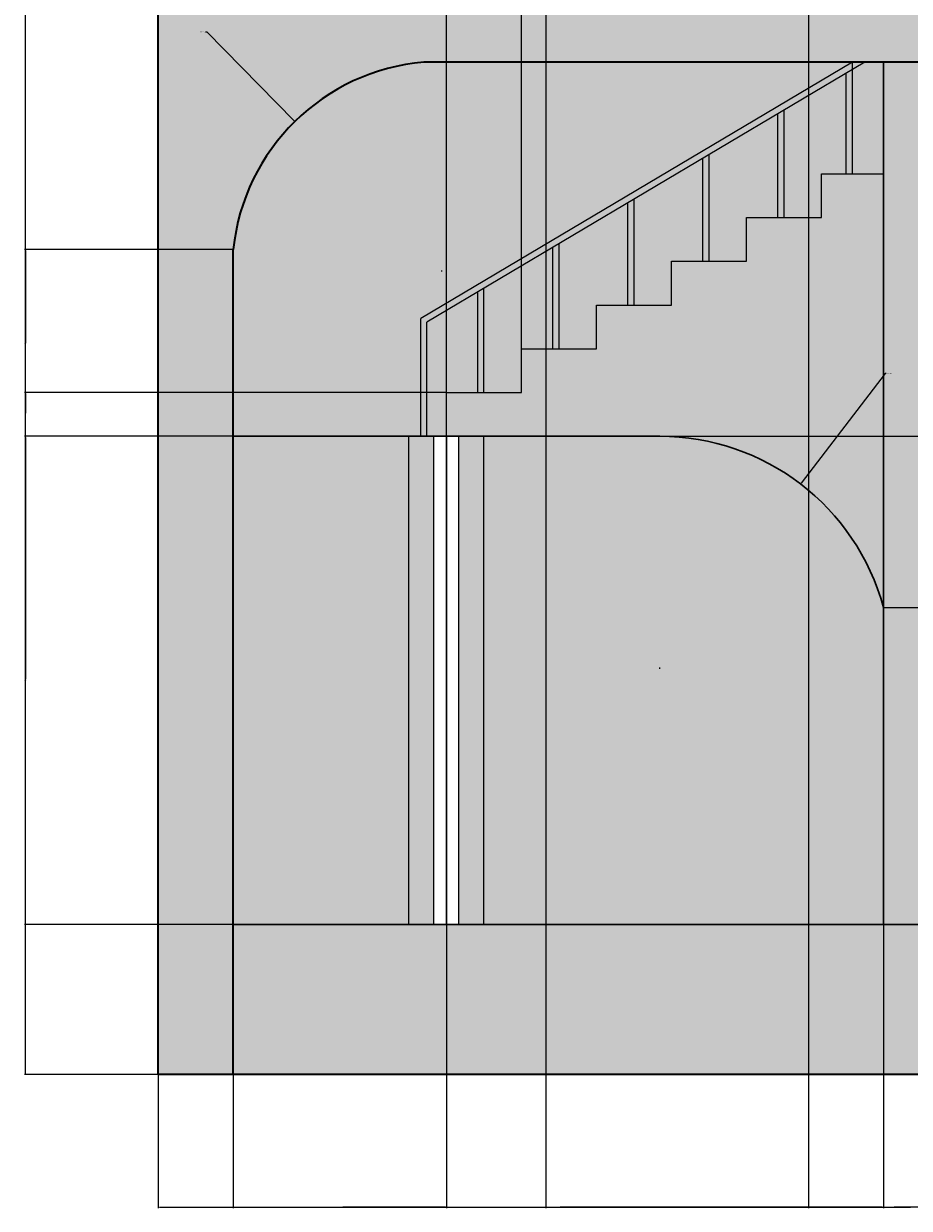
# Model space of a CAD drawing. Units: inches. Extents: x 2051 to 2334, y 814 to 1281.
# Tile 1 of 4: x 2051 to 2193, y 814 to 1003. Entities that reach past the tile are written whole.
import ezdxf

# ---------------------------------------------------------------- set-up
doc = ezdxf.new("R2010")
doc.units = ezdxf.units.IN
for name, color, linetype, lineweight in [('A-ANNO-DIMS', 2, 'Continuous', 18), ('A-COLS', 7, 'Continuous', 30), ('A-ELEV-FRAM', 7, 'Continuous', 35), ('A-ELEV-TRIM', 7, 'Continuous', 18), ('A-FLOR-HRAL', 7, 'Continuous', 18), ('A-FLOR-STRS', 7, 'Continuous', 25), ('A-WALL', 7, 'Continuous', 30)]:
    doc.layers.add(name, color=color, linetype=linetype, lineweight=lineweight)
for name, color, linetype, lineweight, true_color in [('A-ELEV-FRAM-PATT', 251, 'Continuous', 13, 0x636466), ('A-ELEV-INLY-PATT', 18, 'Continuous', 13, 0x000000), ('A-FLOR-HRAL-PATT', 18, 'Continuous', 13, 0x000000), ('A-WALL-PATT', 9, 'Continuous', 13, 0xc7c8ca), ('A-WALL-RECS-PATT', 61, 'Continuous', 13, 0xedee99)]:
    doc.layers.add(name, color=color, linetype=linetype, lineweight=lineweight, true_color=true_color)
doc.styles.get("Standard").update_dxf_attribs({"font": 'arial.ttf'})
doc.dimstyles.get("Standard").update_dxf_attribs({"dimtxt": 0.18, "dimasz": 0.18, "dimexe": 0.18, "dimexo": 0.0625, "dimgap": 0.09, "dimtad": 0, "dimtih": 1, "dimtoh": 1, "dimdec": 4, "dimzin": 0, "dimdsep": 46, "dimtxsty": 'Standard', "dimcen": 0.09, "dimadec": 0, "dimazin": 0, "dimtfac": 1, "dimtdec": 4, "dimtofl": 0, "dimtmove": 0, "dimatfit": 3, "dimfxl": 1, "dimtolj": 1, "dimtzin": 0, "dimarcsym": 0})

# ---------------------------------------------------------------- blocks, each defined once
blk = doc.blocks.new('*D7')
at = {"layer": 'A-ANNO-DIMS', "color": 0, "lineweight": -2, "transparency": 16777216}
for p, q in [((2072.93, 835.18), (2072.93, 813.85)), ((2312.93, 835.18), (2312.93, 813.85)), ((2073.11, 814.03), (2192.64, 814.03)), ((2312.75, 814.03), (2193.22, 814.03))]:
    blk.add_line(p, q, dxfattribs=at)
at = {"layer": 'A-ANNO-DIMS', "color": 0, "transparency": 16777216}
for points in [[(2073.11, 814.06), (2073.11, 814), (2072.93, 814.03)], [(2312.75, 814.06), (2312.75, 814), (2312.93, 814.03)]]:
    blk.add_solid(points, dxfattribs=at)
at = {"layer": 'Defpoints', "color": 0, "transparency": 16777216}
for p in [(2072.93, 835.24), (2312.93, 835.24), (2312.93, 814.03)]:
    blk.add_point(p, dxfattribs=at)
at = {"layer": 'A-ANNO-DIMS', "color": 0, "transparency": 16777216, "insert": (2192.93, 814.03), "char_height": 0.18, "attachment_point": 5}
blk.add_mtext('\\A1;240', dxfattribs=at)
blk = doc.blocks.new('*D8')
at = {"layer": 'A-ANNO-DIMS', "color": 0, "lineweight": -2, "transparency": 16777216}
for p, q in [((2072.87, 1259.24), (2051.53, 1259.24)), ((2051.71, 1259.06), (2051.71, 1047.42)), ((2051.71, 835.42), (2051.71, 1047.06)), ((2072.87, 835.24), (2051.53, 835.24))]:
    blk.add_line(p, q, dxfattribs=at)
at = {"layer": 'A-ANNO-DIMS', "color": 0, "transparency": 16777216}
for points in [[(2051.68, 1259.06), (2051.74, 1259.06), (2051.71, 1259.24)], [(2051.68, 835.42), (2051.74, 835.42), (2051.71, 835.24)]]:
    blk.add_solid(points, dxfattribs=at)
at = {"layer": 'Defpoints', "color": 0, "transparency": 16777216}
for p in [(2051.71, 1259.24), (2072.93, 1259.24), (2072.93, 835.24)]:
    blk.add_point(p, dxfattribs=at)
at = {"layer": 'A-ANNO-DIMS', "color": 0, "transparency": 16777216, "insert": (2051.71, 1047.24), "char_height": 0.18, "attachment_point": 5}
blk.add_mtext('\\A1;424', dxfattribs=at)
blk = doc.blocks.new('*D27')
at = {"layer": 'A-ANNO-DIMS', "color": 0, "lineweight": -2, "transparency": 16777216}
for p, q in [((2134.93, 1063.18), (2134.93, 813.85)), ((2176.93, 1063.18), (2176.93, 813.85)), ((2135.11, 814.03), (2155.71, 814.03)), ((2176.75, 814.03), (2156.15, 814.03))]:
    blk.add_line(p, q, dxfattribs=at)
at = {"layer": 'A-ANNO-DIMS', "color": 0, "transparency": 16777216}
for points in [[(2135.11, 814.06), (2135.11, 814), (2134.93, 814.03)], [(2176.75, 814.06), (2176.75, 814), (2176.93, 814.03)]]:
    blk.add_solid(points, dxfattribs=at)
at = {"layer": 'Defpoints', "color": 0, "transparency": 16777216}
for p in [(2134.93, 1063.24), (2176.93, 1063.24), (2176.93, 814.03)]:
    blk.add_point(p, dxfattribs=at)
at = {"layer": 'A-ANNO-DIMS', "color": 0, "transparency": 16777216, "insert": (2155.93, 814.03), "char_height": 0.18, "attachment_point": 5}
blk.add_mtext('\\A1;42', dxfattribs=at)
blk = doc.blocks.new('*D28')
at = {"layer": 'A-ANNO-DIMS', "color": 0, "lineweight": -2, "transparency": 16777216}
for p, q in [((2203.93, 1065.18), (2203.93, 813.85)), ((2176.93, 1063.18), (2176.93, 813.85)), ((2177.11, 814.03), (2190.21, 814.03)), ((2203.75, 814.03), (2190.65, 814.03))]:
    blk.add_line(p, q, dxfattribs=at)
at = {"layer": 'A-ANNO-DIMS', "color": 0, "transparency": 16777216}
for points in [[(2177.11, 814.06), (2177.11, 814), (2176.93, 814.03)], [(2203.75, 814.06), (2203.75, 814), (2203.93, 814.03)]]:
    blk.add_solid(points, dxfattribs=at)
at = {"layer": 'Defpoints', "color": 0, "transparency": 16777216}
for p in [(2203.93, 1065.24), (2176.93, 1063.24), (2203.93, 814.03)]:
    blk.add_point(p, dxfattribs=at)
at = {"layer": 'A-ANNO-DIMS', "color": 0, "transparency": 16777216, "insert": (2190.43, 814.03), "char_height": 0.18, "attachment_point": 5}
blk.add_mtext('\\A1;27', dxfattribs=at)
blk = doc.blocks.new('*D37')
at = {"layer": 'A-ANNO-DIMS', "color": 0, "lineweight": -2, "transparency": 16777216}
for p, q in [((2084.93, 859.18), (2084.93, 813.85)), ((2188.93, 859.18), (2188.93, 813.85)), ((2085.11, 814.03), (2136.65, 814.03)), ((2188.75, 814.03), (2137.21, 814.03))]:
    blk.add_line(p, q, dxfattribs=at)
at = {"layer": 'A-ANNO-DIMS', "color": 0, "transparency": 16777216}
for points in [[(2085.11, 814.06), (2085.11, 814), (2084.93, 814.03)], [(2188.75, 814.06), (2188.75, 814), (2188.93, 814.03)]]:
    blk.add_solid(points, dxfattribs=at)
at = {"layer": 'Defpoints', "color": 0, "transparency": 16777216}
for p in [(2084.93, 859.24), (2188.93, 859.24), (2188.93, 814.03)]:
    blk.add_point(p, dxfattribs=at)
at = {"layer": 'A-ANNO-DIMS', "color": 0, "transparency": 16777216, "insert": (2136.93, 814.03), "char_height": 0.18, "attachment_point": 5}
blk.add_mtext('\\A1;104', dxfattribs=at)
blk = doc.blocks.new('*D38')
at = {"layer": 'A-ANNO-DIMS', "color": 0, "lineweight": -2, "transparency": 16777216}
for p, q in [((2188.93, 859.18), (2188.93, 813.85)), ((2197.93, 859.18), (2197.93, 813.85)), ((2189.11, 814.03), (2193.28, 814.03)), ((2197.75, 814.03), (2193.58, 814.03))]:
    blk.add_line(p, q, dxfattribs=at)
at = {"layer": 'A-ANNO-DIMS', "color": 0, "transparency": 16777216}
for points in [[(2189.11, 814.06), (2189.11, 814), (2188.93, 814.03)], [(2197.75, 814.06), (2197.75, 814), (2197.93, 814.03)]]:
    blk.add_solid(points, dxfattribs=at)
at = {"layer": 'Defpoints', "color": 0, "transparency": 16777216}
for p in [(2188.93, 859.24), (2197.93, 859.24), (2197.93, 814.03)]:
    blk.add_point(p, dxfattribs=at)
at = {"layer": 'A-ANNO-DIMS', "color": 0, "transparency": 16777216, "insert": (2193.43, 814.03), "char_height": 0.18, "attachment_point": 5}
blk.add_mtext('\\A1;9', dxfattribs=at)
blk = doc.blocks.new('*D40')
at = {"layer": 'A-ANNO-DIMS', "color": 0, "lineweight": -2, "transparency": 16777216}
for p, q in [((2084.87, 937.38), (2051.53, 937.38)), ((2051.71, 937.2), (2051.71, 898.5)), ((2051.71, 859.42), (2051.71, 898.13)), ((2084.87, 859.24), (2051.53, 859.24))]:
    blk.add_line(p, q, dxfattribs=at)
at = {"layer": 'A-ANNO-DIMS', "color": 0, "transparency": 16777216}
for points in [[(2051.68, 937.2), (2051.74, 937.2), (2051.71, 937.38)], [(2051.68, 859.42), (2051.74, 859.42), (2051.71, 859.24)]]:
    blk.add_solid(points, dxfattribs=at)
at = {"layer": 'Defpoints', "color": 0, "transparency": 16777216}
for p in [(2051.71, 937.38), (2084.93, 937.38), (2084.93, 859.24)]:
    blk.add_point(p, dxfattribs=at)
at = {"layer": 'A-ANNO-DIMS', "color": 0, "transparency": 16777216, "insert": (2051.71, 898.31), "char_height": 0.18, "attachment_point": 5}
blk.add_mtext('\\A1;78.14', dxfattribs=at)
blk = doc.blocks.new('*D41')
at = {"layer": 'A-ANNO-DIMS', "color": 0, "lineweight": -2, "transparency": 16777216}
for p, q in [((2084.87, 967.28), (2051.53, 967.28)), ((2051.71, 967.1), (2051.71, 952.52)), ((2051.71, 937.56), (2051.71, 952.15)), ((2084.87, 937.38), (2051.53, 937.38))]:
    blk.add_line(p, q, dxfattribs=at)
at = {"layer": 'A-ANNO-DIMS', "color": 0, "transparency": 16777216}
for points in [[(2051.68, 967.1), (2051.74, 967.1), (2051.71, 967.28)], [(2051.68, 937.56), (2051.74, 937.56), (2051.71, 937.38)]]:
    blk.add_solid(points, dxfattribs=at)
at = {"layer": 'Defpoints', "color": 0, "transparency": 16777216}
for p in [(2051.71, 967.28), (2084.93, 967.28), (2084.93, 937.38)]:
    blk.add_point(p, dxfattribs=at)
at = {"layer": 'A-ANNO-DIMS', "color": 0, "transparency": 16777216, "insert": (2051.71, 952.33), "char_height": 0.18, "attachment_point": 5}
blk.add_mtext('\\A1;29.9', dxfattribs=at)
blk = doc.blocks.new('*D42')
at = {"layer": 'A-ANNO-DIMS', "color": 0, "lineweight": -2, "transparency": 16777216}
for p, q in [((2153.2, 937.38), (2334.32, 937.38)), ((2334.14, 937.2), (2334.14, 923.88)), ((2334.14, 910.18), (2334.14, 923.51)), ((2188.99, 910), (2334.32, 910))]:
    blk.add_line(p, q, dxfattribs=at)
at = {"layer": 'A-ANNO-DIMS', "color": 0, "transparency": 16777216}
for points in [[(2334.11, 937.2), (2334.17, 937.2), (2334.14, 937.38)], [(2334.11, 910.18), (2334.17, 910.18), (2334.14, 910)]]:
    blk.add_solid(points, dxfattribs=at)
at = {"layer": 'Defpoints', "color": 0, "transparency": 16777216}
for p in [(2153.14, 937.38), (2334.14, 937.38), (2188.93, 910)]:
    blk.add_point(p, dxfattribs=at)
at = {"layer": 'A-ANNO-DIMS', "color": 0, "transparency": 16777216, "insert": (2334.14, 923.69), "char_height": 0.18, "attachment_point": 5}
blk.add_mtext('\\A1;27.38', dxfattribs=at)
blk = doc.blocks.new('*D43')
at = {"layer": 'A-ANNO-DIMS', "color": 0, "lineweight": -2, "transparency": 16777216}
for p, q in [((2119.03, 944.45), (2119.03, 1280.64)), ((2119.21, 1280.46), (2124.82, 1280.46)), ((2130.85, 1280.46), (2125.24, 1280.46)), ((2131.03, 944.45), (2131.03, 1280.64))]:
    blk.add_line(p, q, dxfattribs=at)
at = {"layer": 'A-ANNO-DIMS', "color": 0, "transparency": 16777216}
for points in [[(2119.21, 1280.49), (2119.21, 1280.43), (2119.03, 1280.46)], [(2130.85, 1280.49), (2130.85, 1280.43), (2131.03, 1280.46)]]:
    blk.add_solid(points, dxfattribs=at)
at = {"layer": 'Defpoints', "color": 0, "transparency": 16777216}
for p in [(2131.03, 1280.46), (2119.03, 944.38), (2131.03, 944.38)]:
    blk.add_point(p, dxfattribs=at)
at = {"layer": 'A-ANNO-DIMS', "color": 0, "transparency": 16777216, "insert": (2125.03, 1280.46), "char_height": 0.18, "attachment_point": 5}
blk.add_mtext('\\A1;12', dxfattribs=at)
blk = doc.blocks.new('*D44')
at = {"layer": 'A-ANNO-DIMS', "color": 0, "lineweight": -2, "transparency": 16777216}
for p, q in [((2118.9715, 944.383224), (2051.533301, 944.383224)), ((2051.713301, 944.203224), (2051.713301, 941.063224)), ((2051.713301, 937.563224), (2051.713301, 940.703224)), ((2118.9715, 937.383224), (2051.533301, 937.383224))]:
    blk.add_line(p, q, dxfattribs=at)
at = {"layer": 'A-ANNO-DIMS', "color": 0, "transparency": 16777216}
for points in [[(2051.683301, 944.203224), (2051.743301, 944.203224), (2051.713301, 944.383224)], [(2051.683301, 937.563224), (2051.743301, 937.563224), (2051.713301, 937.383224)]]:
    blk.add_solid(points, dxfattribs=at)
at = {"layer": 'Defpoints', "color": 0, "transparency": 16777216}
for p in [(2051.713301, 944.383224), (2119.034, 944.383224), (2119.034, 937.383224)]:
    blk.add_point(p, dxfattribs=at)
at = {"layer": 'A-ANNO-DIMS', "color": 0, "transparency": 16777216, "insert": (2051.713301, 940.883224), "char_height": 0.18, "attachment_point": 5}
blk.add_mtext('\\A1;7', dxfattribs=at)
blk = doc.blocks.new('*D45')
at = {"layer": 'A-ANNO-DIMS', "color": 0, "lineweight": -2, "transparency": 16777216}
for p, q in [((2084.93, 937.32), (2084.93, 813.85)), ((2119.03, 937.32), (2119.03, 813.85)), ((2085.11, 814.03), (2101.52, 814.03)), ((2118.85, 814.03), (2102.44, 814.03))]:
    blk.add_line(p, q, dxfattribs=at)
at = {"layer": 'A-ANNO-DIMS', "color": 0, "transparency": 16777216}
for points in [[(2085.11, 814.06), (2085.11, 814), (2084.93, 814.03)], [(2118.85, 814.06), (2118.85, 814), (2119.03, 814.03)]]:
    blk.add_solid(points, dxfattribs=at)
at = {"layer": 'Defpoints', "color": 0, "transparency": 16777216}
for p in [(2084.93, 937.38), (2119.03, 937.38), (2119.03, 814.03)]:
    blk.add_point(p, dxfattribs=at)
at = {"layer": 'A-ANNO-DIMS', "color": 0, "transparency": 16777216, "insert": (2101.98, 814.03), "char_height": 0.18, "attachment_point": 5}
blk.add_mtext('\\A1;34.106', dxfattribs=at)
blk = doc.blocks.new('*D61')
at = {"layer": 'A-ANNO-DIMS', "color": 0, "lineweight": -2, "transparency": 16777216}
for p, q in [((2189.19, 947.42), (2175.78, 929.9)), ((2189.37, 947.42), (2189.19, 947.42)), ((2153.14, 900.21), (2153.14, 900.39)), ((2153.05, 900.3), (2153.23, 900.3))]:
    blk.add_line(p, q, dxfattribs=at)
at = {"layer": 'A-ANNO-DIMS', "color": 0, "transparency": 16777216}
blk.add_solid([(2175.76, 929.91), (2175.8, 929.88), (2175.67, 929.75)], dxfattribs=at)
at = {"layer": 'Defpoints', "color": 0, "transparency": 16777216}
for p in [(2175.67, 929.75), (2153.14, 900.3)]:
    blk.add_point(p, dxfattribs=at)
at = {"layer": 'A-ANNO-DIMS', "color": 0, "transparency": 16777216, "insert": (2189.85, 947.42), "char_height": 0.18, "attachment_point": 5}
blk.add_mtext('\\A1;R37.08', dxfattribs=at)
blk = doc.blocks.new('*D62')
at = {"layer": 'A-ANNO-DIMS', "color": 0, "lineweight": -2, "transparency": 16777216}
for p, q in [((2080.5, 1002.1), (2080.68, 1002.1)), ((2080.68, 1002.1), (2094.65, 987.88)), ((2118.18, 963.84), (2118.36, 963.84)), ((2118.27, 963.75), (2118.27, 963.93))]:
    blk.add_line(p, q, dxfattribs=at)
at = {"layer": 'A-ANNO-DIMS', "color": 0, "transparency": 16777216}
blk.add_solid([(2094.68, 987.9), (2094.63, 987.86), (2094.78, 987.76)], dxfattribs=at)
at = {"layer": 'Defpoints', "color": 0, "transparency": 16777216}
for p in [(2094.78, 987.76), (2118.27, 963.84)]:
    blk.add_point(p, dxfattribs=at)
at = {"layer": 'A-ANNO-DIMS', "color": 0, "transparency": 16777216, "insert": (2080.02, 1002.1), "char_height": 0.18, "attachment_point": 5}
blk.add_mtext('\\A1;R33.52', dxfattribs=at)

msp = doc.modelspace()

# ---------------------------------------------------------------- hatches: boundary and pattern name
at = {"layer": 'A-ELEV-FRAM-PATT'}
h = msp.add_hatch(color=256, dxfattribs=at)
h.dxf.hatch_style = 1
h.paths.add_polyline_path([(2312.9283, 1217.2439), (2303.9283, 1217.2439), (2303.9283, 1059.2439, -0.29083376), (2256.3338, 1017.2439), (2110.9283, 1017.2439, -0.41949346), (2084.9283, 1039.0559), (2084.9283, 1221.9535, -0.37464242), (2110.9283, 1247.2439), (2247.6639, 1247.2439), (2247.6639, 1259.2439), (2072.9283, 1259.2439), (2072.9283, 835.2439), (2084.9283, 835.2439), (2084.9283, 967.2832, -0.36016597), (2115.4224, 997.2439), (2312.9283, 997.2439)])
h = msp.add_hatch(color=256, dxfattribs=at)
h.dxf.hatch_style = 1
h.paths.add_polyline_path([(2312.9283, 997.2439), (2303.9283, 997.2439), (2303.9283, 859.2439), (2312.9283, 859.2439)])
h.paths.add_polyline_path([(2197.9283, 997.2439), (2188.9283, 997.2439), (2188.9283, 859.2439), (2197.9283, 859.2439)])
h = msp.add_hatch(color=256, dxfattribs=at)
h.dxf.hatch_style = 1
h.paths.add_polyline_path([(2312.9283, 859.2439), (2084.9283, 859.2439), (2084.9283, 835.2439), (2312.9283, 835.2439)])
at = {"layer": 'A-ELEV-INLY-PATT'}
h = msp.add_hatch(color=256, dxfattribs=at)
h.dxf.hatch_style = 1
h.paths.add_polyline_path([(2125.034, 937.3832), (2121.034, 937.3832), (2121.034, 859.2439), (2125.034, 859.2439)])
h.paths.add_polyline_path([(2117.034, 937.3832), (2113.034, 937.3832), (2113.034, 859.2439), (2117.034, 859.2439)])
at = {"layer": 'A-FLOR-HRAL-PATT'}
h = msp.add_hatch(color=256, dxfattribs=at)
h.dxf.hatch_style = 1
h.paths.add_polyline_path([(2183.9812, 996.0809), (2183.9812, 997.2439), (2114.9154, 956.236), (2114.9154, 937.3832), (2115.9154, 937.3832), (2115.9154, 955.6667)])
h.paths.add_polyline_path([(2185.9399, 997.2439), (2183.9812, 997.2439), (2183.9812, 996.0809)])
h.paths.add_polyline_path([(2183.9812, 996.0809), (2182.9812, 995.4872), (2182.9812, 979.3832), (2183.9812, 979.3832)], flags=17)
h.paths.add_polyline_path([(2173.034, 989.581), (2172.034, 988.9873), (2172.034, 972.3832), (2173.034, 972.3832)], flags=17)
h.paths.add_polyline_path([(2161.034, 982.456), (2160.034, 981.8622), (2160.034, 965.3832), (2161.034, 965.3832)], flags=17)
h.paths.add_polyline_path([(2149.034, 975.331), (2148.034, 974.7372), (2148.034, 958.3832), (2149.034, 958.3832)], flags=17)
h.paths.add_polyline_path([(2137.034, 968.2059), (2136.034, 967.6122), (2136.034, 951.3832), (2137.034, 951.3832)], flags=17)
h.paths.add_polyline_path([(2125.034, 961.0809), (2124.034, 960.4872), (2124.034, 944.3832), (2125.034, 944.3832)], flags=17)
at = {"layer": 'A-WALL-PATT'}
h = msp.add_hatch(color=256, dxfattribs=at)
h.dxf.hatch_style = 1
h.paths.add_polyline_path([(2188.9283, 910.0037, 0.33864929), (2153.1397, 937.3832), (2125.034, 937.3832), (2125.034, 859.2439), (2188.9283, 859.2439)])
h.paths.add_polyline_path([(2113.034, 937.3832), (2084.9283, 937.3832), (2084.9283, 859.2439), (2113.034, 859.2439)])
h.paths.add_polyline_path([(2312.9283, 859.2439), (2084.9283, 859.2439), (2084.9283, 835.2439), (2312.9283, 835.2439)])
h.paths.add_polyline_path([(2288.9283, 1123.0714), (2288.9283, 1065.2439), (2303.9283, 1065.2439), (2303.9283, 1175.2439), (2176.9283, 1175.2439), (2176.9283, 1065.2439), (2203.9283, 1065.2439), (2203.9283, 1123.0714, -0.93632991)])
h.paths.add_polyline_path([(2197.9283, 1247.2439), (2112.9283, 1247.2439), (2112.9283, 1217.2439), (2197.9283, 1217.2439)])
h.paths.add_polyline_path([(2110.9283, 1247.2439, 0.11468321), (2098.9283, 1243.754), (2098.9283, 1019.2065, 0.12996728), (2110.9283, 1017.2439)])
h.paths.add_polyline_path([(2096.9283, 1242.5167, 0.22673474), (2084.9283, 1221.9535), (2084.9283, 1039.0559, 0.24937907), (2096.9283, 1020.2168)])
at = {"layer": 'A-WALL-RECS-PATT'}
h = msp.add_hatch(color=256, dxfattribs=at)
h.dxf.hatch_style = 1
h.paths.add_polyline_path([(2188.9283, 979.3832), (2179.034, 979.3832), (2179.034, 972.3832), (2167.034, 972.3832), (2167.034, 965.3832), (2155.034, 965.3832), (2155.034, 958.3832), (2143.034, 958.3832), (2143.034, 951.3832), (2131.034, 951.3832), (2131.034, 944.3832), (2119.034, 944.3832), (2119.034, 937.3832), (2153.1397, 937.3832, -0.33864929), (2188.9283, 910.0037)])
h.paths.add_polyline_path([(2183.9812, 997.2439), (2115.4224, 997.2439, 0.36016597), (2084.9283, 967.2832), (2084.9283, 937.3832), (2114.9154, 937.3832), (2114.9154, 956.236)])
h.paths.add_polyline_path([(2124.034, 960.4872), (2115.9154, 955.6667), (2115.9154, 937.3832), (2119.034, 937.3832), (2119.034, 944.3832), (2124.034, 944.3832)], flags=17)
h.paths.add_polyline_path([(2136.034, 967.6122), (2125.034, 961.0809), (2125.034, 944.3832), (2131.034, 944.3832), (2131.034, 951.3832), (2136.034, 951.3832)], flags=17)
h.paths.add_polyline_path([(2148.034, 974.7372), (2137.034, 968.2059), (2137.034, 951.3832), (2143.034, 951.3832), (2143.034, 958.3832), (2148.034, 958.3832)], flags=17)
h.paths.add_polyline_path([(2160.034, 981.8622), (2149.034, 975.331), (2149.034, 958.3832), (2155.034, 958.3832), (2155.034, 965.3832), (2160.034, 965.3832)], flags=17)
h.paths.add_polyline_path([(2172.034, 988.9873), (2161.034, 982.456), (2161.034, 965.3832), (2167.034, 965.3832), (2167.034, 972.3832), (2172.034, 972.3832)], flags=17)
h.paths.add_polyline_path([(2182.9812, 995.4872), (2173.034, 989.581), (2173.034, 972.3832), (2179.034, 972.3832), (2179.034, 979.3832), (2182.9812, 979.3832)], flags=17)
h.paths.add_polyline_path([(2188.9283, 997.2439), (2183.9812, 997.2439), (2183.9812, 979.3832), (2188.9283, 979.3832)])

# ---------------------------------------------------------------- linework, layer by layer
at = {"layer": 'A-COLS'}
msp.add_line((2188.9283, 859.2439), (2188.9283, 997.2439), dxfattribs=at)
at = {"layer": 'A-ELEV-FRAM'}
for p, q in [((2072.9283, 835.2439), (2072.9283, 1259.2439)), ((2312.9283, 997.2439), (2115.4224, 997.2439)), ((2084.9283, 835.2439), (2084.9283, 967.2832)), ((2312.9283, 835.2439), (2072.9283, 835.2439))]:
    msp.add_line(p, q, dxfattribs=at)
msp.add_arc((2118.2741, 963.8426), 33.5228, 94.879894, 174.109071, dxfattribs=at)
at = {"layer": 'A-ELEV-TRIM'}
for p, q in [((2113.034, 859.2439), (2113.034, 937.3832)), ((2117.034, 859.2439), (2117.034, 937.3832)), ((2119.034, 859.2439), (2119.034, 937.3832)), ((2121.034, 859.2439), (2121.034, 937.3832)), ((2125.034, 859.2439), (2125.034, 937.3832))]:
    msp.add_line(p, q, dxfattribs=at)
at = {"layer": 'A-FLOR-HRAL'}
for p, q in [((2183.9812, 997.2439), (2114.9154, 956.236)), ((2185.9399, 997.2439), (2115.9154, 955.6667)), ((2183.9812, 979.3832), (2183.9812, 997.2439)), ((2182.9812, 979.3832), (2182.9812, 995.4872)), ((2173.034, 972.3832), (2173.034, 989.581)), ((2172.034, 972.3832), (2172.034, 988.9873)), ((2161.034, 965.3832), (2161.034, 982.456)), ((2160.034, 965.3832), (2160.034, 981.8622)), ((2148.034, 958.3832), (2148.034, 974.7372)), ((2149.034, 958.3832), (2149.034, 975.331)), ((2136.034, 951.3832), (2136.034, 967.6122)), ((2137.034, 951.3832), (2137.034, 968.2059)), ((2125.034, 944.3832), (2125.034, 961.0809)), ((2124.034, 944.3832), (2124.034, 960.4872)), ((2114.9154, 937.3832), (2114.9154, 956.236)), ((2115.9154, 937.3832), (2115.9154, 955.6667))]:
    msp.add_line(p, q, dxfattribs=at)
at = {"layer": 'A-FLOR-STRS'}
for p, q in [((2179.034, 972.3832), (2179.034, 979.3832)), ((2179.034, 979.3832), (2188.9283, 979.3832)), ((2167.034, 965.3832), (2167.034, 972.3832)), ((2167.034, 972.3832), (2179.034, 972.3832)), ((2155.034, 958.3832), (2155.034, 965.3832)), ((2155.034, 965.3832), (2167.034, 965.3832)), ((2143.034, 951.3832), (2143.034, 958.3832)), ((2143.034, 958.3832), (2155.034, 958.3832)), ((2131.034, 944.3832), (2131.034, 951.3832)), ((2131.034, 951.3832), (2143.034, 951.3832)), ((2119.034, 937.3832), (2119.034, 944.3832)), ((2119.034, 944.3832), (2131.034, 944.3832))]:
    msp.add_line(p, q, dxfattribs=at)
at = {"layer": 'A-WALL'}
for p, q in [((2153.1397, 937.3832), (2084.9283, 937.3832)), ((2312.9283, 859.2439), (2084.9283, 859.2439))]:
    msp.add_line(p, q, dxfattribs=at)
msp.add_arc((2153.1397, 900.3033), 37.0799, 15.165463, 90, dxfattribs=at)

# ---------------------------------------------------------------- dimensions: what is measured, and where the dimension line sits
at = {"layer": 'A-ANNO-DIMS'}
for base, p1, p2, override, picture, middle in [((2131.034, 1280.4589), (2119.034, 944.3832), (2131.034, 944.3832), {"dimdec": 0, "dimlfac": 1, "dimrnd": 0, "dimzin": 0, "dimdsep": 46, "dimlunit": 2}, '*D43', (2125.034, 1280.4589)), ((2203.9283, 814.0289), (2176.9283, 1063.2439), (2203.9283, 1065.2439), {"dimdec": 0, "dimlfac": 1, "dimrnd": 0, "dimzin": 0, "dimdsep": 46, "dimlunit": 2}, '*D28', (2190.4283, 814.0289)), ((2176.9283, 814.0289), (2134.9283, 1063.2439), (2176.9283, 1063.2439), {"dimdec": 0, "dimlfac": 1, "dimrnd": 0, "dimzin": 0, "dimdsep": 46, "dimlunit": 2}, '*D27', (2155.9283, 814.0289)), ((2119.034, 814.0289), (2084.9283, 937.3832), (2119.034, 937.3832), {"dimdec": 3, "dimlfac": 1, "dimrnd": 0, "dimzin": 0, "dimdsep": 46, "dimlunit": 2}, '*D45', (2101.9812, 814.0289)), ((2188.9283, 814.0289), (2084.9283, 859.2439), (2188.9283, 859.2439), {"dimdec": 0, "dimlfac": 1, "dimrnd": 0, "dimzin": 0, "dimdsep": 46, "dimlunit": 2}, '*D37', (2136.9283, 814.0289)), ((2197.9283, 814.0289), (2188.9283, 859.2439), (2197.9283, 859.2439), {"dimdec": 0, "dimlfac": 1, "dimrnd": 0, "dimzin": 0, "dimdsep": 46, "dimlunit": 2}, '*D38', (2193.4283, 814.0289)), ((2312.9283, 814.0289), (2072.9283, 835.2439), (2312.9283, 835.2439), {"dimdec": 0, "dimlfac": 1, "dimrnd": 0, "dimzin": 0, "dimdsep": 46, "dimlunit": 2}, '*D7', (2192.9283, 814.0289))]:
    dim = msp.add_linear_dim(base=base, p1=p1, p2=p2, dimstyle='Standard', override=override, dxfattribs=at)
    dim.commit()
    dim.dimension.update_dxf_attribs({"geometry": picture, "text_midpoint": middle})
for base, p1, p2, override, picture, middle in [((2051.7133, 1259.2439), (2072.9283, 835.2439), (2072.9283, 1259.2439), {"dimdec": 0, "dimlfac": 1, "dimrnd": 0, "dimzin": 0, "dimdsep": 46, "dimlunit": 2}, '*D8', (2051.7133, 1047.2439)), ((2051.7133, 967.2832), (2084.9283, 937.3832), (2084.9283, 967.2832), {"dimdec": 1, "dimlfac": 1, "dimrnd": 0, "dimzin": 0, "dimdsep": 46, "dimlunit": 2}, '*D41', (2051.7133, 952.3332)), ((2051.7133, 944.3832), (2119.034, 937.3832), (2119.034, 944.3832), {"dimdec": 0, "dimlfac": 1, "dimrnd": 0, "dimzin": 0, "dimdsep": 46, "dimlunit": 2}, '*D44', (2051.7133, 940.8832)), ((2051.7133, 937.3832), (2084.9283, 859.2439), (2084.9283, 937.3832), {"dimdec": 2, "dimlfac": 1, "dimrnd": 0, "dimzin": 0, "dimdsep": 46, "dimlunit": 2}, '*D40', (2051.7133, 898.3136)), ((2334.1433, 937.3832), (2188.9283, 910.0037), (2153.1397, 937.3832), {"dimdec": 2, "dimlfac": 1, "dimrnd": 0, "dimzin": 0, "dimdsep": 46, "dimlunit": 2}, '*D42', (2334.1433, 923.6934))]:
    dim = msp.add_linear_dim(base=base, p1=p1, p2=p2, angle=90, dimstyle='Standard', override=override, dxfattribs=at)
    dim.commit()
    dim.dimension.update_dxf_attribs({"geometry": picture, "text_midpoint": middle})
for center, mpoint, picture, middle in [((2118.2741, 963.8426), (2094.78, 987.755), '*D62', (2080.0246, 1002.1025)), ((2153.1397, 900.3033), (2175.6702, 929.7532), '*D61', (2189.8485, 947.4232))]:
    dim = msp.add_radius_dim(center=center, mpoint=mpoint, dimstyle='Standard', override={"dimdec": 2, "dimlfac": 1, "dimrnd": 0, "dimzin": 0, "dimdsep": 46, "dimlunit": 2}, dxfattribs=at)
    dim.commit()
    dim.dimension.update_dxf_attribs({"geometry": picture, "text_midpoint": middle, "dimtype": 164})

doc.saveas('drawing.dxf')
